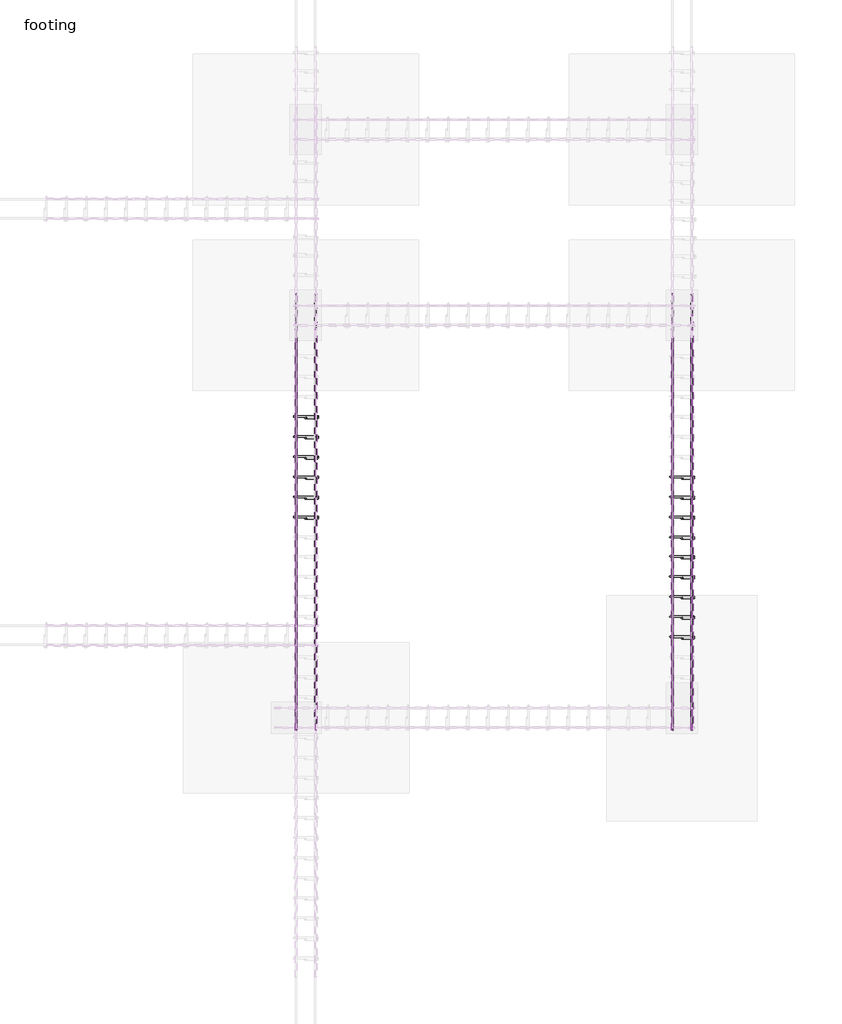
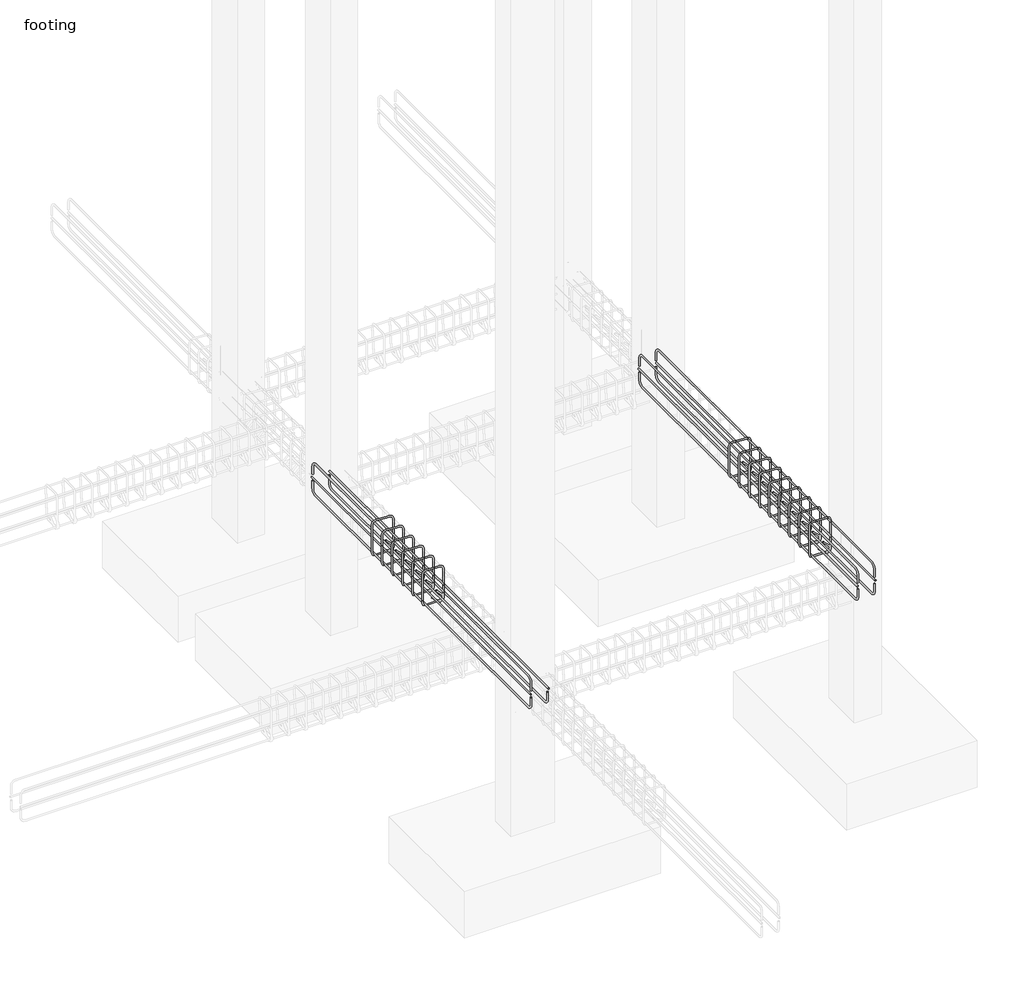
# One storey, part 12 of 21: 26 reinforcing bars.
"""IFC4 building model written with IfcOpenShell, lengths in millimetres."""

from ifc_helpers import new_model, si_unit, point, frame, origin, place, context, project, spatial, polyline, circle_curve, trimmed, segment, composite_curve, element, save
from ifc_brep_helpers import swept_disk

model = new_model("IFC4")

# Units and contexts
model_context = context("Model", 3, world=origin())
ifc_project = project(units=[si_unit("LENGTHUNIT", "METRE", prefix="MILLI")], contexts=[model_context])

# Site, building, storey
site = spatial("IfcSite", under=ifc_project)
building = spatial("IfcBuilding", under=site)
storey = spatial("IfcBuildingStorey", under=building, Name="footing", Elevation=-1524.0)

# Reinforcing bars
placement = place(None, origin())
element("IfcReinforcingBar", 1, at=placement, inside=storey, context=model_context, shape_type="SolidModel", body=[
    swept_disk(composite_curve([segment(polyline([(-7943.5663014, 3342.0730744, -170.2827408), (-7943.5663014, 3342.0730744, -94.0827408)]), True, "CONTINUOUS"), segment(trimmed(circle_curve(frame((-7943.5663014, 3386.5230744, -94.0827408), z_axis=(-1.0, 0.0, 0.0), x_axis=(0.0, -44.44999999999982, 0.0)), 44.45), [point((-7943.5663014, 3342.0730744, -94.0827408))], [point((-7943.5663014, 3386.5230744, -49.6327408))], True, "CARTESIAN"), True, "CONTINUOUS"), segment(polyline([(-7943.5663014, 3386.5230744, -49.6327408), (-7943.5663014, 6822.6668244, -49.6327408)]), True, "CONTINUOUS"), segment(trimmed(circle_curve(frame((-7943.5663014, 6822.6668244, -94.0827408), z_axis=(-1.0, 0.0, 0.0), x_axis=(0.0, 0.0, 44.449999999999996)), 44.45), [point((-7943.5663014, 6822.6668244, -49.6327408))], [point((-7943.5663014, 6867.1168244, -94.0827408))], True, "CARTESIAN"), True, "CONTINUOUS"), segment(polyline([(-7943.5663014, 6867.1168244, -94.0827408), (-7943.5663014, 6867.1168244, -170.2827408)]), True, "CONTINUOUS")], self_intersect=False), 6.35),
])
element("IfcReinforcingBar", 2, at=placement, inside=storey, context=model_context, shape_type="SolidModel", body=[
    swept_disk(composite_curve([segment(polyline([(-7788.8317831, 3342.0730744, -236.1172592), (-7788.8317831, 3342.0730744, -312.3172592)]), True, "CONTINUOUS"), segment(trimmed(circle_curve(frame((-7788.8317831, 3386.5230744, -312.3172592), z_axis=(1.0, 0.0, 0.0), x_axis=(0.0, -44.44999999999982, 0.0)), 44.45), [point((-7788.8317831, 3342.0730744, -312.3172592))], [point((-7788.8317831, 3386.5230744, -356.7672592))], True, "CARTESIAN"), True, "CONTINUOUS"), segment(polyline([(-7788.8317831, 3386.5230744, -356.7672592), (-7788.8317831, 6822.6668244, -356.7672592)]), True, "CONTINUOUS"), segment(trimmed(circle_curve(frame((-7788.8317831, 6822.6668244, -312.3172592), z_axis=(1.0, 0.0, 0.0), x_axis=(0.0, 0.0, -44.44999999999999)), 44.45), [point((-7788.8317831, 6822.6668244, -356.7672592))], [point((-7788.8317831, 6867.1168244, -312.3172592))], True, "CARTESIAN"), True, "CONTINUOUS"), segment(polyline([(-7788.8317831, 6867.1168244, -312.3172592), (-7788.8317831, 6867.1168244, -236.1172592)]), True, "CONTINUOUS")], self_intersect=False), 6.35),
])
element("IfcReinforcingBar", 3, at=placement, inside=storey, context=model_context, shape_type="SolidModel", body=[
    swept_disk(composite_curve([segment(polyline([(-7943.5663014, 3342.0730744, -236.1172592), (-7943.5663014, 3342.0730744, -312.3172592)]), True, "CONTINUOUS"), segment(trimmed(circle_curve(frame((-7943.5663014, 3386.5230744, -312.3172592), z_axis=(1.0, 0.0, 0.0), x_axis=(0.0, -44.44999999999982, 0.0)), 44.45), [point((-7943.5663014, 3342.0730744, -312.3172592))], [point((-7943.5663014, 3386.5230744, -356.7672592))], True, "CARTESIAN"), True, "CONTINUOUS"), segment(polyline([(-7943.5663014, 3386.5230744, -356.7672592), (-7943.5663014, 6822.6668244, -356.7672592)]), True, "CONTINUOUS"), segment(trimmed(circle_curve(frame((-7943.5663014, 6822.6668244, -312.3172592), z_axis=(1.0, 0.0, 0.0), x_axis=(0.0, 0.0, -44.44999999999999)), 44.45), [point((-7943.5663014, 6822.6668244, -356.7672592))], [point((-7943.5663014, 6867.1168244, -312.3172592))], True, "CARTESIAN"), True, "CONTINUOUS"), segment(polyline([(-7943.5663014, 6867.1168244, -312.3172592), (-7943.5663014, 6867.1168244, -236.1172592)]), True, "CONTINUOUS")], self_intersect=False), 6.35),
])
element("IfcReinforcingBar", 4, at=placement, inside=storey, context=model_context, shape_type="SolidModel", body=[
    swept_disk(composite_curve([segment(polyline([(-7783.2521673, 3335.7230744, -203.2), (-7783.2521673, 6873.4668244, -203.2)]), True, "CONTINUOUS")], self_intersect=False), 6.35),
])
element("IfcReinforcingBar", 5, at=placement, inside=storey, context=model_context, shape_type="SolidModel", body=[
    swept_disk(composite_curve([segment(polyline([(-7949.1459173, 3335.7230744, -203.2), (-7949.1459173, 6873.4668244, -203.2)]), True, "CONTINUOUS")], self_intersect=False), 6.35),
])
element("IfcReinforcingBar", 6, at=placement, inside=storey, context=model_context, shape_type="SolidModel", body=[
    swept_disk(composite_curve([segment(polyline([(-7834.7165254, 5064.2456073, -265.9812362), (-7779.851527, 5064.2456073, -320.8462347)]), True, "CONTINUOUS"), segment(trimmed(circle_curve(frame((-7802.3021673, 5064.2456073, -343.296875), z_axis=(0.0, 1.0, 0.0), x_axis=(22.450640300000487, 0.0, 22.450640299999975)), 31.75), [point((-7779.851527, 5064.2456073, -320.8462347))], [point((-7802.3021673, 5064.2456073, -375.046875))], True, "CARTESIAN"), True, "CONTINUOUS"), segment(polyline([(-7802.3021673, 5064.2456073, -375.046875), (-7930.0959173, 5064.2456073, -375.046875)]), True, "CONTINUOUS"), segment(trimmed(circle_curve(frame((-7930.0959173, 5064.2456073, -343.296875), z_axis=(0.0, 1.0, 0.0), x_axis=(0.0, 0.0, -31.75)), 31.75), [point((-7930.0959173, 5064.2456073, -375.046875))], [point((-7961.8459173, 5064.2456073, -343.296875))], True, "CARTESIAN"), True, "CONTINUOUS"), segment(polyline([(-7961.8459173, 5064.2456073, -343.296875), (-7961.8459173, 5064.2456073, -63.103125)]), True, "CONTINUOUS"), segment(trimmed(circle_curve(frame((-7930.165658, 5062.1423536, -63.103125), z_axis=(0.0662442117686417, 0.9978034397651431, 0.0), x_axis=(-31.680259300000216, 2.1032537000000957, 0.0)), 31.75), [point((-7961.8459173, 5064.2456073, -63.103125))], [point((-7930.165658, 5062.1423536, -31.353125))], True, "CARTESIAN"), True, "CONTINUOUS"), segment(polyline([(-7930.165658, 5062.1423536, -31.353125), (-7802.2324265, 5053.648861, -31.353125)]), True, "CONTINUOUS"), segment(trimmed(circle_curve(frame((-7802.2324265, 5053.648861, -63.103125), z_axis=(0.06624421176864169, 0.997803439765143, 0.0), x_axis=(0.0, 0.0, 31.75)), 31.75), [point((-7802.2324265, 5053.648861, -31.353125))], [point((-7770.5521673, 5051.5456073, -63.103125))], True, "CARTESIAN"), True, "CONTINUOUS"), segment(polyline([(-7770.5521673, 5051.5456073, -63.103125), (-7770.5521673, 5051.5456073, -343.296875)]), True, "CONTINUOUS"), segment(trimmed(circle_curve(frame((-7802.3021673, 5051.5456073, -343.296875), z_axis=(0.0, 1.0, 0.0), x_axis=(31.75, 0.0, 0.0)), 31.75), [point((-7770.5521673, 5051.5456073, -343.296875))], [point((-7824.7528076, 5051.5456073, -365.7475153))], True, "CARTESIAN"), True, "CONTINUOUS"), segment(polyline([(-7824.7528076, 5051.5456073, -365.7475153), (-7879.617806, 5051.5456073, -310.8825168)]), True, "CONTINUOUS")], self_intersect=False), 6.35),
])
element("IfcReinforcingBar", 7, at=placement, inside=storey, context=model_context, shape_type="SolidModel", body=[
    swept_disk(composite_curve([segment(polyline([(-7834.7165254, 5226.9456073, -265.9812362), (-7779.851527, 5226.9456073, -320.8462347)]), True, "CONTINUOUS"), segment(trimmed(circle_curve(frame((-7802.3021673, 5226.9456073, -343.296875), z_axis=(0.0, 1.0, 0.0), x_axis=(22.450640300000487, 0.0, 22.450640299999975)), 31.75), [point((-7779.851527, 5226.9456073, -320.8462347))], [point((-7802.3021673, 5226.9456073, -375.046875))], True, "CARTESIAN"), True, "CONTINUOUS"), segment(polyline([(-7802.3021673, 5226.9456073, -375.046875), (-7930.0959173, 5226.9456073, -375.046875)]), True, "CONTINUOUS"), segment(trimmed(circle_curve(frame((-7930.0959173, 5226.9456073, -343.296875), z_axis=(0.0, 1.0, 0.0), x_axis=(0.0, 0.0, -31.75)), 31.75), [point((-7930.0959173, 5226.9456073, -375.046875))], [point((-7961.8459173, 5226.9456073, -343.296875))], True, "CARTESIAN"), True, "CONTINUOUS"), segment(polyline([(-7961.8459173, 5226.9456073, -343.296875), (-7961.8459173, 5226.9456073, -63.103125)]), True, "CONTINUOUS"), segment(trimmed(circle_curve(frame((-7930.165658, 5224.8423536, -63.103125), z_axis=(0.0662442117686417, 0.9978034397651431, 0.0), x_axis=(-31.680259300000216, 2.1032537000000957, 0.0)), 31.75), [point((-7961.8459173, 5226.9456073, -63.103125))], [point((-7930.165658, 5224.8423536, -31.353125))], True, "CARTESIAN"), True, "CONTINUOUS"), segment(polyline([(-7930.165658, 5224.8423536, -31.353125), (-7802.2324265, 5216.348861, -31.353125)]), True, "CONTINUOUS"), segment(trimmed(circle_curve(frame((-7802.2324265, 5216.348861, -63.103125), z_axis=(0.06624421176864169, 0.997803439765143, 0.0), x_axis=(0.0, 0.0, 31.75)), 31.75), [point((-7802.2324265, 5216.348861, -31.353125))], [point((-7770.5521673, 5214.2456073, -63.103125))], True, "CARTESIAN"), True, "CONTINUOUS"), segment(polyline([(-7770.5521673, 5214.2456073, -63.103125), (-7770.5521673, 5214.2456073, -343.296875)]), True, "CONTINUOUS"), segment(trimmed(circle_curve(frame((-7802.3021673, 5214.2456073, -343.296875), z_axis=(0.0, 1.0, 0.0), x_axis=(31.75, 0.0, 0.0)), 31.75), [point((-7770.5521673, 5214.2456073, -343.296875))], [point((-7824.7528076, 5214.2456073, -365.7475153))], True, "CARTESIAN"), True, "CONTINUOUS"), segment(polyline([(-7824.7528076, 5214.2456073, -365.7475153), (-7879.617806, 5214.2456073, -310.8825168)]), True, "CONTINUOUS")], self_intersect=False), 6.35),
])
element("IfcReinforcingBar", 8, at=placement, inside=storey, context=model_context, shape_type="SolidModel", body=[
    swept_disk(composite_curve([segment(polyline([(-7834.7165254, 5389.6456073, -265.9812362), (-7779.851527, 5389.6456073, -320.8462347)]), True, "CONTINUOUS"), segment(trimmed(circle_curve(frame((-7802.3021673, 5389.6456073, -343.296875), z_axis=(0.0, 1.0, 0.0), x_axis=(22.450640300000487, 0.0, 22.450640299999975)), 31.75), [point((-7779.851527, 5389.6456073, -320.8462347))], [point((-7802.3021673, 5389.6456073, -375.046875))], True, "CARTESIAN"), True, "CONTINUOUS"), segment(polyline([(-7802.3021673, 5389.6456073, -375.046875), (-7930.0959173, 5389.6456073, -375.046875)]), True, "CONTINUOUS"), segment(trimmed(circle_curve(frame((-7930.0959173, 5389.6456073, -343.296875), z_axis=(0.0, 1.0, 0.0), x_axis=(0.0, 0.0, -31.75)), 31.75), [point((-7930.0959173, 5389.6456073, -375.046875))], [point((-7961.8459173, 5389.6456073, -343.296875))], True, "CARTESIAN"), True, "CONTINUOUS"), segment(polyline([(-7961.8459173, 5389.6456073, -343.296875), (-7961.8459173, 5389.6456073, -63.103125)]), True, "CONTINUOUS"), segment(trimmed(circle_curve(frame((-7930.165658, 5387.5423536, -63.103125), z_axis=(0.0662442117686417, 0.9978034397651431, 0.0), x_axis=(-31.680259300000216, 2.1032537000000957, 0.0)), 31.75), [point((-7961.8459173, 5389.6456073, -63.103125))], [point((-7930.165658, 5387.5423536, -31.353125))], True, "CARTESIAN"), True, "CONTINUOUS"), segment(polyline([(-7930.165658, 5387.5423536, -31.353125), (-7802.2324265, 5379.048861, -31.353125)]), True, "CONTINUOUS"), segment(trimmed(circle_curve(frame((-7802.2324265, 5379.048861, -63.103125), z_axis=(0.06624421176864169, 0.997803439765143, 0.0), x_axis=(0.0, 0.0, 31.75)), 31.75), [point((-7802.2324265, 5379.048861, -31.353125))], [point((-7770.5521673, 5376.9456073, -63.103125))], True, "CARTESIAN"), True, "CONTINUOUS"), segment(polyline([(-7770.5521673, 5376.9456073, -63.103125), (-7770.5521673, 5376.9456073, -343.296875)]), True, "CONTINUOUS"), segment(trimmed(circle_curve(frame((-7802.3021673, 5376.9456073, -343.296875), z_axis=(0.0, 1.0, 0.0), x_axis=(31.75, 0.0, 0.0)), 31.75), [point((-7770.5521673, 5376.9456073, -343.296875))], [point((-7824.7528076, 5376.9456073, -365.7475153))], True, "CARTESIAN"), True, "CONTINUOUS"), segment(polyline([(-7824.7528076, 5376.9456073, -365.7475153), (-7879.617806, 5376.9456073, -310.8825168)]), True, "CONTINUOUS")], self_intersect=False), 6.35),
])
element("IfcReinforcingBar", 9, at=placement, inside=storey, context=model_context, shape_type="SolidModel", body=[
    swept_disk(composite_curve([segment(polyline([(-7834.7165254, 5552.3456073, -265.9812362), (-7779.851527, 5552.3456073, -320.8462347)]), True, "CONTINUOUS"), segment(trimmed(circle_curve(frame((-7802.3021673, 5552.3456073, -343.296875), z_axis=(0.0, 1.0, 0.0), x_axis=(22.450640300000487, 0.0, 22.450640299999975)), 31.75), [point((-7779.851527, 5552.3456073, -320.8462347))], [point((-7802.3021673, 5552.3456073, -375.046875))], True, "CARTESIAN"), True, "CONTINUOUS"), segment(polyline([(-7802.3021673, 5552.3456073, -375.046875), (-7930.0959173, 5552.3456073, -375.046875)]), True, "CONTINUOUS"), segment(trimmed(circle_curve(frame((-7930.0959173, 5552.3456073, -343.296875), z_axis=(0.0, 1.0, 0.0), x_axis=(0.0, 0.0, -31.75)), 31.75), [point((-7930.0959173, 5552.3456073, -375.046875))], [point((-7961.8459173, 5552.3456073, -343.296875))], True, "CARTESIAN"), True, "CONTINUOUS"), segment(polyline([(-7961.8459173, 5552.3456073, -343.296875), (-7961.8459173, 5552.3456073, -63.103125)]), True, "CONTINUOUS"), segment(trimmed(circle_curve(frame((-7930.165658, 5550.2423536, -63.103125), z_axis=(0.0662442117686417, 0.9978034397651431, 0.0), x_axis=(-31.680259300000216, 2.1032537000000957, 0.0)), 31.75), [point((-7961.8459173, 5552.3456073, -63.103125))], [point((-7930.165658, 5550.2423536, -31.353125))], True, "CARTESIAN"), True, "CONTINUOUS"), segment(polyline([(-7930.165658, 5550.2423536, -31.353125), (-7802.2324265, 5541.748861, -31.353125)]), True, "CONTINUOUS"), segment(trimmed(circle_curve(frame((-7802.2324265, 5541.748861, -63.103125), z_axis=(0.06624421176864169, 0.997803439765143, 0.0), x_axis=(0.0, 0.0, 31.75)), 31.75), [point((-7802.2324265, 5541.748861, -31.353125))], [point((-7770.5521673, 5539.6456073, -63.103125))], True, "CARTESIAN"), True, "CONTINUOUS"), segment(polyline([(-7770.5521673, 5539.6456073, -63.103125), (-7770.5521673, 5539.6456073, -343.296875)]), True, "CONTINUOUS"), segment(trimmed(circle_curve(frame((-7802.3021673, 5539.6456073, -343.296875), z_axis=(0.0, 1.0, 0.0), x_axis=(31.75, 0.0, 0.0)), 31.75), [point((-7770.5521673, 5539.6456073, -343.296875))], [point((-7824.7528076, 5539.6456073, -365.7475153))], True, "CARTESIAN"), True, "CONTINUOUS"), segment(polyline([(-7824.7528076, 5539.6456073, -365.7475153), (-7879.617806, 5539.6456073, -310.8825168)]), True, "CONTINUOUS")], self_intersect=False), 6.35),
])
element("IfcReinforcingBar", 10, at=placement, inside=storey, context=model_context, shape_type="SolidModel", body=[
    swept_disk(composite_curve([segment(polyline([(-7834.7165254, 5715.0456073, -265.9812362), (-7779.851527, 5715.0456073, -320.8462347)]), True, "CONTINUOUS"), segment(trimmed(circle_curve(frame((-7802.3021673, 5715.0456073, -343.296875), z_axis=(0.0, 1.0, 0.0), x_axis=(22.450640300000487, 0.0, 22.450640299999975)), 31.75), [point((-7779.851527, 5715.0456073, -320.8462347))], [point((-7802.3021673, 5715.0456073, -375.046875))], True, "CARTESIAN"), True, "CONTINUOUS"), segment(polyline([(-7802.3021673, 5715.0456073, -375.046875), (-7930.0959173, 5715.0456073, -375.046875)]), True, "CONTINUOUS"), segment(trimmed(circle_curve(frame((-7930.0959173, 5715.0456073, -343.296875), z_axis=(0.0, 1.0, 0.0), x_axis=(0.0, 0.0, -31.75)), 31.75), [point((-7930.0959173, 5715.0456073, -375.046875))], [point((-7961.8459173, 5715.0456073, -343.296875))], True, "CARTESIAN"), True, "CONTINUOUS"), segment(polyline([(-7961.8459173, 5715.0456073, -343.296875), (-7961.8459173, 5715.0456073, -63.103125)]), True, "CONTINUOUS"), segment(trimmed(circle_curve(frame((-7930.165658, 5712.9423536, -63.103125), z_axis=(0.0662442117686417, 0.9978034397651431, 0.0), x_axis=(-31.680259300000216, 2.103253699999186, 0.0)), 31.75), [point((-7961.8459173, 5715.0456073, -63.103125))], [point((-7930.165658, 5712.9423536, -31.353125))], True, "CARTESIAN"), True, "CONTINUOUS"), segment(polyline([(-7930.165658, 5712.9423536, -31.353125), (-7802.2324265, 5704.448861, -31.353125)]), True, "CONTINUOUS"), segment(trimmed(circle_curve(frame((-7802.2324265, 5704.448861, -63.103125), z_axis=(0.06624421176864169, 0.997803439765143, 0.0), x_axis=(0.0, 0.0, 31.75)), 31.75), [point((-7802.2324265, 5704.448861, -31.353125))], [point((-7770.5521673, 5702.3456073, -63.103125))], True, "CARTESIAN"), True, "CONTINUOUS"), segment(polyline([(-7770.5521673, 5702.3456073, -63.103125), (-7770.5521673, 5702.3456073, -343.296875)]), True, "CONTINUOUS"), segment(trimmed(circle_curve(frame((-7802.3021673, 5702.3456073, -343.296875), z_axis=(0.0, 1.0, 0.0), x_axis=(31.75, 0.0, 0.0)), 31.75), [point((-7770.5521673, 5702.3456073, -343.296875))], [point((-7824.7528076, 5702.3456073, -365.7475153))], True, "CARTESIAN"), True, "CONTINUOUS"), segment(polyline([(-7824.7528076, 5702.3456073, -365.7475153), (-7879.617806, 5702.3456073, -310.8825168)]), True, "CONTINUOUS")], self_intersect=False), 6.35),
])
element("IfcReinforcingBar", 11, at=placement, inside=storey, context=model_context, shape_type="SolidModel", body=[
    swept_disk(composite_curve([segment(polyline([(-7834.7165254, 5877.7456073, -265.9812362), (-7779.851527, 5877.7456073, -320.8462347)]), True, "CONTINUOUS"), segment(trimmed(circle_curve(frame((-7802.3021673, 5877.7456073, -343.296875), z_axis=(0.0, 1.0, 0.0), x_axis=(22.450640300000487, 0.0, 22.450640299999975)), 31.75), [point((-7779.851527, 5877.7456073, -320.8462347))], [point((-7802.3021673, 5877.7456073, -375.046875))], True, "CARTESIAN"), True, "CONTINUOUS"), segment(polyline([(-7802.3021673, 5877.7456073, -375.046875), (-7930.0959173, 5877.7456073, -375.046875)]), True, "CONTINUOUS"), segment(trimmed(circle_curve(frame((-7930.0959173, 5877.7456073, -343.296875), z_axis=(0.0, 1.0, 0.0), x_axis=(0.0, 0.0, -31.75)), 31.75), [point((-7930.0959173, 5877.7456073, -375.046875))], [point((-7961.8459173, 5877.7456073, -343.296875))], True, "CARTESIAN"), True, "CONTINUOUS"), segment(polyline([(-7961.8459173, 5877.7456073, -343.296875), (-7961.8459173, 5877.7456073, -63.103125)]), True, "CONTINUOUS"), segment(trimmed(circle_curve(frame((-7930.165658, 5875.6423536, -63.103125), z_axis=(0.0662442117686417, 0.9978034397651431, 0.0), x_axis=(-31.680259300000216, 2.1032537000000957, 0.0)), 31.75), [point((-7961.8459173, 5877.7456073, -63.103125))], [point((-7930.165658, 5875.6423536, -31.353125))], True, "CARTESIAN"), True, "CONTINUOUS"), segment(polyline([(-7930.165658, 5875.6423536, -31.353125), (-7802.2324265, 5867.148861, -31.353125)]), True, "CONTINUOUS"), segment(trimmed(circle_curve(frame((-7802.2324265, 5867.148861, -63.103125), z_axis=(0.06624421176864169, 0.997803439765143, 0.0), x_axis=(0.0, 0.0, 31.75)), 31.75), [point((-7802.2324265, 5867.148861, -31.353125))], [point((-7770.5521673, 5865.0456073, -63.103125))], True, "CARTESIAN"), True, "CONTINUOUS"), segment(polyline([(-7770.5521673, 5865.0456073, -63.103125), (-7770.5521673, 5865.0456073, -343.296875)]), True, "CONTINUOUS"), segment(trimmed(circle_curve(frame((-7802.3021673, 5865.0456073, -343.296875), z_axis=(0.0, 1.0, 0.0), x_axis=(31.75, 0.0, 0.0)), 31.75), [point((-7770.5521673, 5865.0456073, -343.296875))], [point((-7824.7528076, 5865.0456073, -365.7475153))], True, "CARTESIAN"), True, "CONTINUOUS"), segment(polyline([(-7824.7528076, 5865.0456073, -365.7475153), (-7879.617806, 5865.0456073, -310.8825168)]), True, "CONTINUOUS")], self_intersect=False), 6.35),
])
element("IfcReinforcingBar", 12, at=placement, inside=storey, context=model_context, shape_type="SolidModel", body=[
    swept_disk(composite_curve([segment(polyline([(-4740.8317831, 3342.0730744, -170.2827408), (-4740.8317831, 3342.0730744, -94.0827408)]), True, "CONTINUOUS"), segment(trimmed(circle_curve(frame((-4740.8317831, 3386.5230744, -94.0827408), z_axis=(-1.0, 0.0, 0.0), x_axis=(0.0, -44.44999999999982, 0.0)), 44.45), [point((-4740.8317831, 3342.0730744, -94.0827408))], [point((-4740.8317831, 3386.5230744, -49.6327408))], True, "CARTESIAN"), True, "CONTINUOUS"), segment(polyline([(-4740.8317831, 3386.5230744, -49.6327408), (-4740.8317831, 6822.6668244, -49.6327408)]), True, "CONTINUOUS"), segment(trimmed(circle_curve(frame((-4740.8317831, 6822.6668244, -94.0827408), z_axis=(-1.0, 0.0, 0.0), x_axis=(0.0, 0.0, 44.449999999999996)), 44.45), [point((-4740.8317831, 6822.6668244, -49.6327408))], [point((-4740.8317831, 6867.1168244, -94.0827408))], True, "CARTESIAN"), True, "CONTINUOUS"), segment(polyline([(-4740.8317831, 6867.1168244, -94.0827408), (-4740.8317831, 6867.1168244, -170.2827408)]), True, "CONTINUOUS")], self_intersect=False), 6.35),
])
element("IfcReinforcingBar", 13, at=placement, inside=storey, context=model_context, shape_type="SolidModel", body=[
    swept_disk(composite_curve([segment(polyline([(-4895.5663014, 3342.0730744, -170.2827408), (-4895.5663014, 3342.0730744, -94.0827408)]), True, "CONTINUOUS"), segment(trimmed(circle_curve(frame((-4895.5663014, 3386.5230744, -94.0827408), z_axis=(-1.0, 0.0, 0.0), x_axis=(0.0, -44.44999999999982, 0.0)), 44.45), [point((-4895.5663014, 3342.0730744, -94.0827408))], [point((-4895.5663014, 3386.5230744, -49.6327408))], True, "CARTESIAN"), True, "CONTINUOUS"), segment(polyline([(-4895.5663014, 3386.5230744, -49.6327408), (-4895.5663014, 6822.6668244, -49.6327408)]), True, "CONTINUOUS"), segment(trimmed(circle_curve(frame((-4895.5663014, 6822.6668244, -94.0827408), z_axis=(-1.0, 0.0, 0.0), x_axis=(0.0, 0.0, 44.449999999999996)), 44.45), [point((-4895.5663014, 6822.6668244, -49.6327408))], [point((-4895.5663014, 6867.1168244, -94.0827408))], True, "CARTESIAN"), True, "CONTINUOUS"), segment(polyline([(-4895.5663014, 6867.1168244, -94.0827408), (-4895.5663014, 6867.1168244, -170.2827408)]), True, "CONTINUOUS")], self_intersect=False), 6.35),
])
element("IfcReinforcingBar", 14, at=placement, inside=storey, context=model_context, shape_type="SolidModel", body=[
    swept_disk(composite_curve([segment(polyline([(-4740.8317831, 3342.0730744, -236.1172592), (-4740.8317831, 3342.0730744, -312.3172592)]), True, "CONTINUOUS"), segment(trimmed(circle_curve(frame((-4740.8317831, 3386.5230744, -312.3172592), z_axis=(1.0, 0.0, 0.0), x_axis=(0.0, -44.44999999999982, 0.0)), 44.45), [point((-4740.8317831, 3342.0730744, -312.3172592))], [point((-4740.8317831, 3386.5230744, -356.7672592))], True, "CARTESIAN"), True, "CONTINUOUS"), segment(polyline([(-4740.8317831, 3386.5230744, -356.7672592), (-4740.8317831, 6822.6668244, -356.7672592)]), True, "CONTINUOUS"), segment(trimmed(circle_curve(frame((-4740.8317831, 6822.6668244, -312.3172592), z_axis=(1.0, 0.0, 0.0), x_axis=(0.0, 0.0, -44.44999999999999)), 44.45), [point((-4740.8317831, 6822.6668244, -356.7672592))], [point((-4740.8317831, 6867.1168244, -312.3172592))], True, "CARTESIAN"), True, "CONTINUOUS"), segment(polyline([(-4740.8317831, 6867.1168244, -312.3172592), (-4740.8317831, 6867.1168244, -236.1172592)]), True, "CONTINUOUS")], self_intersect=False), 6.35),
])
element("IfcReinforcingBar", 15, at=placement, inside=storey, context=model_context, shape_type="SolidModel", body=[
    swept_disk(composite_curve([segment(polyline([(-4895.5663014, 3342.0730744, -236.1172592), (-4895.5663014, 3342.0730744, -312.3172592)]), True, "CONTINUOUS"), segment(trimmed(circle_curve(frame((-4895.5663014, 3386.5230744, -312.3172592), z_axis=(1.0, 0.0, 0.0), x_axis=(0.0, -44.44999999999982, 0.0)), 44.45), [point((-4895.5663014, 3342.0730744, -312.3172592))], [point((-4895.5663014, 3386.5230744, -356.7672592))], True, "CARTESIAN"), True, "CONTINUOUS"), segment(polyline([(-4895.5663014, 3386.5230744, -356.7672592), (-4895.5663014, 6822.6668244, -356.7672592)]), True, "CONTINUOUS"), segment(trimmed(circle_curve(frame((-4895.5663014, 6822.6668244, -312.3172592), z_axis=(1.0, 0.0, 0.0), x_axis=(0.0, 0.0, -44.44999999999999)), 44.45), [point((-4895.5663014, 6822.6668244, -356.7672592))], [point((-4895.5663014, 6867.1168244, -312.3172592))], True, "CARTESIAN"), True, "CONTINUOUS"), segment(polyline([(-4895.5663014, 6867.1168244, -312.3172592), (-4895.5663014, 6867.1168244, -236.1172592)]), True, "CONTINUOUS")], self_intersect=False), 6.35),
])
element("IfcReinforcingBar", 16, at=placement, inside=storey, context=model_context, shape_type="SolidModel", body=[
    swept_disk(composite_curve([segment(polyline([(-4735.2521673, 3335.7230744, -203.2), (-4735.2521673, 6873.4668244, -203.2)]), True, "CONTINUOUS")], self_intersect=False), 6.35),
])
element("IfcReinforcingBar", 17, at=placement, inside=storey, context=model_context, shape_type="SolidModel", body=[
    swept_disk(composite_curve([segment(polyline([(-4901.1459173, 3335.7230744, -203.2), (-4901.1459173, 6873.4668244, -203.2)]), True, "CONTINUOUS")], self_intersect=False), 6.35),
])
element("IfcReinforcingBar", 18, at=placement, inside=storey, context=model_context, shape_type="SolidModel", body=[
    swept_disk(composite_curve([segment(polyline([(-4786.7165254, 4094.3956073, -265.9812362), (-4731.851527, 4094.3956073, -320.8462347)]), True, "CONTINUOUS"), segment(trimmed(circle_curve(frame((-4754.3021673, 4094.3956073, -343.296875), z_axis=(0.0, 1.0, 0.0), x_axis=(22.450640300000487, 0.0, 22.450640299999975)), 31.75), [point((-4731.851527, 4094.3956073, -320.8462347))], [point((-4754.3021673, 4094.3956073, -375.046875))], True, "CARTESIAN"), True, "CONTINUOUS"), segment(polyline([(-4754.3021673, 4094.3956073, -375.046875), (-4882.0959173, 4094.3956073, -375.046875)]), True, "CONTINUOUS"), segment(trimmed(circle_curve(frame((-4882.0959173, 4094.3956073, -343.296875), z_axis=(0.0, 1.0, 0.0), x_axis=(0.0, 0.0, -31.75)), 31.75), [point((-4882.0959173, 4094.3956073, -375.046875))], [point((-4913.8459173, 4094.3956073, -343.296875))], True, "CARTESIAN"), True, "CONTINUOUS"), segment(polyline([(-4913.8459173, 4094.3956073, -343.296875), (-4913.8459173, 4094.3956073, -63.103125)]), True, "CONTINUOUS"), segment(trimmed(circle_curve(frame((-4882.165658, 4092.2923536, -63.103125), z_axis=(0.0662442117686417, 0.9978034397651431, 0.0), x_axis=(-31.680259300000216, 2.1032537000000957, 0.0)), 31.75), [point((-4913.8459173, 4094.3956073, -63.103125))], [point((-4882.165658, 4092.2923536, -31.353125))], True, "CARTESIAN"), True, "CONTINUOUS"), segment(polyline([(-4882.165658, 4092.2923536, -31.353125), (-4754.2324265, 4083.798861, -31.353125)]), True, "CONTINUOUS"), segment(trimmed(circle_curve(frame((-4754.2324265, 4083.798861, -63.103125), z_axis=(0.06624421176864169, 0.997803439765143, 0.0), x_axis=(0.0, 0.0, 31.75)), 31.75), [point((-4754.2324265, 4083.798861, -31.353125))], [point((-4722.5521673, 4081.6956073, -63.103125))], True, "CARTESIAN"), True, "CONTINUOUS"), segment(polyline([(-4722.5521673, 4081.6956073, -63.103125), (-4722.5521673, 4081.6956073, -343.296875)]), True, "CONTINUOUS"), segment(trimmed(circle_curve(frame((-4754.3021673, 4081.6956073, -343.296875), z_axis=(0.0, 1.0, 0.0), x_axis=(31.75, 0.0, 0.0)), 31.75), [point((-4722.5521673, 4081.6956073, -343.296875))], [point((-4776.7528076, 4081.6956073, -365.7475153))], True, "CARTESIAN"), True, "CONTINUOUS"), segment(polyline([(-4776.7528076, 4081.6956073, -365.7475153), (-4831.617806, 4081.6956073, -310.8825168)]), True, "CONTINUOUS")], self_intersect=False), 6.35),
])
element("IfcReinforcingBar", 19, at=placement, inside=storey, context=model_context, shape_type="SolidModel", body=[
    swept_disk(composite_curve([segment(polyline([(-4786.7165254, 4257.0956073, -265.9812362), (-4731.851527, 4257.0956073, -320.8462347)]), True, "CONTINUOUS"), segment(trimmed(circle_curve(frame((-4754.3021673, 4257.0956073, -343.296875), z_axis=(0.0, 1.0, 0.0), x_axis=(22.450640300000487, 0.0, 22.450640299999975)), 31.75), [point((-4731.851527, 4257.0956073, -320.8462347))], [point((-4754.3021673, 4257.0956073, -375.046875))], True, "CARTESIAN"), True, "CONTINUOUS"), segment(polyline([(-4754.3021673, 4257.0956073, -375.046875), (-4882.0959173, 4257.0956073, -375.046875)]), True, "CONTINUOUS"), segment(trimmed(circle_curve(frame((-4882.0959173, 4257.0956073, -343.296875), z_axis=(0.0, 1.0, 0.0), x_axis=(0.0, 0.0, -31.75)), 31.75), [point((-4882.0959173, 4257.0956073, -375.046875))], [point((-4913.8459173, 4257.0956073, -343.296875))], True, "CARTESIAN"), True, "CONTINUOUS"), segment(polyline([(-4913.8459173, 4257.0956073, -343.296875), (-4913.8459173, 4257.0956073, -63.103125)]), True, "CONTINUOUS"), segment(trimmed(circle_curve(frame((-4882.165658, 4254.9923536, -63.103125), z_axis=(0.0662442117686417, 0.9978034397651431, 0.0), x_axis=(-31.680259300000216, 2.1032537000000957, 0.0)), 31.75), [point((-4913.8459173, 4257.0956073, -63.103125))], [point((-4882.165658, 4254.9923536, -31.353125))], True, "CARTESIAN"), True, "CONTINUOUS"), segment(polyline([(-4882.165658, 4254.9923536, -31.353125), (-4754.2324265, 4246.498861, -31.353125)]), True, "CONTINUOUS"), segment(trimmed(circle_curve(frame((-4754.2324265, 4246.498861, -63.103125), z_axis=(0.06624421176864169, 0.997803439765143, 0.0), x_axis=(0.0, 0.0, 31.75)), 31.75), [point((-4754.2324265, 4246.498861, -31.353125))], [point((-4722.5521673, 4244.3956073, -63.103125))], True, "CARTESIAN"), True, "CONTINUOUS"), segment(polyline([(-4722.5521673, 4244.3956073, -63.103125), (-4722.5521673, 4244.3956073, -343.296875)]), True, "CONTINUOUS"), segment(trimmed(circle_curve(frame((-4754.3021673, 4244.3956073, -343.296875), z_axis=(0.0, 1.0, 0.0), x_axis=(31.75, 0.0, 0.0)), 31.75), [point((-4722.5521673, 4244.3956073, -343.296875))], [point((-4776.7528076, 4244.3956073, -365.7475153))], True, "CARTESIAN"), True, "CONTINUOUS"), segment(polyline([(-4776.7528076, 4244.3956073, -365.7475153), (-4831.617806, 4244.3956073, -310.8825168)]), True, "CONTINUOUS")], self_intersect=False), 6.35),
])
element("IfcReinforcingBar", 20, at=placement, inside=storey, context=model_context, shape_type="SolidModel", body=[
    swept_disk(composite_curve([segment(polyline([(-4786.7165254, 4419.7956073, -265.9812362), (-4731.851527, 4419.7956073, -320.8462347)]), True, "CONTINUOUS"), segment(trimmed(circle_curve(frame((-4754.3021673, 4419.7956073, -343.296875), z_axis=(0.0, 1.0, 0.0), x_axis=(22.450640300000487, 0.0, 22.450640299999975)), 31.75), [point((-4731.851527, 4419.7956073, -320.8462347))], [point((-4754.3021673, 4419.7956073, -375.046875))], True, "CARTESIAN"), True, "CONTINUOUS"), segment(polyline([(-4754.3021673, 4419.7956073, -375.046875), (-4882.0959173, 4419.7956073, -375.046875)]), True, "CONTINUOUS"), segment(trimmed(circle_curve(frame((-4882.0959173, 4419.7956073, -343.296875), z_axis=(0.0, 1.0, 0.0), x_axis=(0.0, 0.0, -31.75)), 31.75), [point((-4882.0959173, 4419.7956073, -375.046875))], [point((-4913.8459173, 4419.7956073, -343.296875))], True, "CARTESIAN"), True, "CONTINUOUS"), segment(polyline([(-4913.8459173, 4419.7956073, -343.296875), (-4913.8459173, 4419.7956073, -63.103125)]), True, "CONTINUOUS"), segment(trimmed(circle_curve(frame((-4882.165658, 4417.6923536, -63.103125), z_axis=(0.0662442117686417, 0.9978034397651431, 0.0), x_axis=(-31.680259300000216, 2.103253699999186, 0.0)), 31.75), [point((-4913.8459173, 4419.7956073, -63.103125))], [point((-4882.165658, 4417.6923536, -31.353125))], True, "CARTESIAN"), True, "CONTINUOUS"), segment(polyline([(-4882.165658, 4417.6923536, -31.353125), (-4754.2324265, 4409.198861, -31.353125)]), True, "CONTINUOUS"), segment(trimmed(circle_curve(frame((-4754.2324265, 4409.198861, -63.103125), z_axis=(0.06624421176864169, 0.997803439765143, 0.0), x_axis=(0.0, 0.0, 31.75)), 31.75), [point((-4754.2324265, 4409.198861, -31.353125))], [point((-4722.5521673, 4407.0956073, -63.103125))], True, "CARTESIAN"), True, "CONTINUOUS"), segment(polyline([(-4722.5521673, 4407.0956073, -63.103125), (-4722.5521673, 4407.0956073, -343.296875)]), True, "CONTINUOUS"), segment(trimmed(circle_curve(frame((-4754.3021673, 4407.0956073, -343.296875), z_axis=(0.0, 1.0, 0.0), x_axis=(31.75, 0.0, 0.0)), 31.75), [point((-4722.5521673, 4407.0956073, -343.296875))], [point((-4776.7528076, 4407.0956073, -365.7475153))], True, "CARTESIAN"), True, "CONTINUOUS"), segment(polyline([(-4776.7528076, 4407.0956073, -365.7475153), (-4831.617806, 4407.0956073, -310.8825168)]), True, "CONTINUOUS")], self_intersect=False), 6.35),
])
element("IfcReinforcingBar", 21, at=placement, inside=storey, context=model_context, shape_type="SolidModel", body=[
    swept_disk(composite_curve([segment(polyline([(-4786.7165254, 4582.4956073, -265.9812362), (-4731.851527, 4582.4956073, -320.8462347)]), True, "CONTINUOUS"), segment(trimmed(circle_curve(frame((-4754.3021673, 4582.4956073, -343.296875), z_axis=(0.0, 1.0, 0.0), x_axis=(22.450640300000487, 0.0, 22.450640299999975)), 31.75), [point((-4731.851527, 4582.4956073, -320.8462347))], [point((-4754.3021673, 4582.4956073, -375.046875))], True, "CARTESIAN"), True, "CONTINUOUS"), segment(polyline([(-4754.3021673, 4582.4956073, -375.046875), (-4882.0959173, 4582.4956073, -375.046875)]), True, "CONTINUOUS"), segment(trimmed(circle_curve(frame((-4882.0959173, 4582.4956073, -343.296875), z_axis=(0.0, 1.0, 0.0), x_axis=(0.0, 0.0, -31.75)), 31.75), [point((-4882.0959173, 4582.4956073, -375.046875))], [point((-4913.8459173, 4582.4956073, -343.296875))], True, "CARTESIAN"), True, "CONTINUOUS"), segment(polyline([(-4913.8459173, 4582.4956073, -343.296875), (-4913.8459173, 4582.4956073, -63.103125)]), True, "CONTINUOUS"), segment(trimmed(circle_curve(frame((-4882.165658, 4580.3923536, -63.103125), z_axis=(0.0662442117686417, 0.9978034397651431, 0.0), x_axis=(-31.680259300000216, 2.1032537000000957, 0.0)), 31.75), [point((-4913.8459173, 4582.4956073, -63.103125))], [point((-4882.165658, 4580.3923536, -31.353125))], True, "CARTESIAN"), True, "CONTINUOUS"), segment(polyline([(-4882.165658, 4580.3923536, -31.353125), (-4754.2324265, 4571.898861, -31.353125)]), True, "CONTINUOUS"), segment(trimmed(circle_curve(frame((-4754.2324265, 4571.898861, -63.103125), z_axis=(0.06624421176864169, 0.997803439765143, 0.0), x_axis=(0.0, 0.0, 31.75)), 31.75), [point((-4754.2324265, 4571.898861, -31.353125))], [point((-4722.5521673, 4569.7956073, -63.103125))], True, "CARTESIAN"), True, "CONTINUOUS"), segment(polyline([(-4722.5521673, 4569.7956073, -63.103125), (-4722.5521673, 4569.7956073, -343.296875)]), True, "CONTINUOUS"), segment(trimmed(circle_curve(frame((-4754.3021673, 4569.7956073, -343.296875), z_axis=(0.0, 1.0, 0.0), x_axis=(31.75, 0.0, 0.0)), 31.75), [point((-4722.5521673, 4569.7956073, -343.296875))], [point((-4776.7528076, 4569.7956073, -365.7475153))], True, "CARTESIAN"), True, "CONTINUOUS"), segment(polyline([(-4776.7528076, 4569.7956073, -365.7475153), (-4831.617806, 4569.7956073, -310.8825168)]), True, "CONTINUOUS")], self_intersect=False), 6.35),
])
element("IfcReinforcingBar", 22, at=placement, inside=storey, context=model_context, shape_type="SolidModel", body=[
    swept_disk(composite_curve([segment(polyline([(-4786.7165254, 4745.1956073, -265.9812362), (-4731.851527, 4745.1956073, -320.8462347)]), True, "CONTINUOUS"), segment(trimmed(circle_curve(frame((-4754.3021673, 4745.1956073, -343.296875), z_axis=(0.0, 1.0, 0.0), x_axis=(22.450640300000487, 0.0, 22.450640299999975)), 31.75), [point((-4731.851527, 4745.1956073, -320.8462347))], [point((-4754.3021673, 4745.1956073, -375.046875))], True, "CARTESIAN"), True, "CONTINUOUS"), segment(polyline([(-4754.3021673, 4745.1956073, -375.046875), (-4882.0959173, 4745.1956073, -375.046875)]), True, "CONTINUOUS"), segment(trimmed(circle_curve(frame((-4882.0959173, 4745.1956073, -343.296875), z_axis=(0.0, 1.0, 0.0), x_axis=(0.0, 0.0, -31.75)), 31.75), [point((-4882.0959173, 4745.1956073, -375.046875))], [point((-4913.8459173, 4745.1956073, -343.296875))], True, "CARTESIAN"), True, "CONTINUOUS"), segment(polyline([(-4913.8459173, 4745.1956073, -343.296875), (-4913.8459173, 4745.1956073, -63.103125)]), True, "CONTINUOUS"), segment(trimmed(circle_curve(frame((-4882.165658, 4743.0923536, -63.103125), z_axis=(0.0662442117686417, 0.9978034397651431, 0.0), x_axis=(-31.680259300000216, 2.1032537000000957, 0.0)), 31.75), [point((-4913.8459173, 4745.1956073, -63.103125))], [point((-4882.165658, 4743.0923536, -31.353125))], True, "CARTESIAN"), True, "CONTINUOUS"), segment(polyline([(-4882.165658, 4743.0923536, -31.353125), (-4754.2324265, 4734.598861, -31.353125)]), True, "CONTINUOUS"), segment(trimmed(circle_curve(frame((-4754.2324265, 4734.598861, -63.103125), z_axis=(0.06624421176864169, 0.997803439765143, 0.0), x_axis=(0.0, 0.0, 31.75)), 31.75), [point((-4754.2324265, 4734.598861, -31.353125))], [point((-4722.5521673, 4732.4956073, -63.103125))], True, "CARTESIAN"), True, "CONTINUOUS"), segment(polyline([(-4722.5521673, 4732.4956073, -63.103125), (-4722.5521673, 4732.4956073, -343.296875)]), True, "CONTINUOUS"), segment(trimmed(circle_curve(frame((-4754.3021673, 4732.4956073, -343.296875), z_axis=(0.0, 1.0, 0.0), x_axis=(31.75, 0.0, 0.0)), 31.75), [point((-4722.5521673, 4732.4956073, -343.296875))], [point((-4776.7528076, 4732.4956073, -365.7475153))], True, "CARTESIAN"), True, "CONTINUOUS"), segment(polyline([(-4776.7528076, 4732.4956073, -365.7475153), (-4831.617806, 4732.4956073, -310.8825168)]), True, "CONTINUOUS")], self_intersect=False), 6.35),
])
element("IfcReinforcingBar", 23, at=placement, inside=storey, context=model_context, shape_type="SolidModel", body=[
    swept_disk(composite_curve([segment(polyline([(-4786.7165254, 4901.5456073, -265.9812362), (-4731.851527, 4901.5456073, -320.8462347)]), True, "CONTINUOUS"), segment(trimmed(circle_curve(frame((-4754.3021673, 4901.5456073, -343.296875), z_axis=(0.0, 1.0, 0.0), x_axis=(22.450640300000487, 0.0, 22.450640299999975)), 31.75), [point((-4731.851527, 4901.5456073, -320.8462347))], [point((-4754.3021673, 4901.5456073, -375.046875))], True, "CARTESIAN"), True, "CONTINUOUS"), segment(polyline([(-4754.3021673, 4901.5456073, -375.046875), (-4882.0959173, 4901.5456073, -375.046875)]), True, "CONTINUOUS"), segment(trimmed(circle_curve(frame((-4882.0959173, 4901.5456073, -343.296875), z_axis=(0.0, 1.0, 0.0), x_axis=(0.0, 0.0, -31.75)), 31.75), [point((-4882.0959173, 4901.5456073, -375.046875))], [point((-4913.8459173, 4901.5456073, -343.296875))], True, "CARTESIAN"), True, "CONTINUOUS"), segment(polyline([(-4913.8459173, 4901.5456073, -343.296875), (-4913.8459173, 4901.5456073, -63.103125)]), True, "CONTINUOUS"), segment(trimmed(circle_curve(frame((-4882.165658, 4899.4423536, -63.103125), z_axis=(0.0662442117686417, 0.9978034397651431, 0.0), x_axis=(-31.680259300000216, 2.103253699999186, 0.0)), 31.75), [point((-4913.8459173, 4901.5456073, -63.103125))], [point((-4882.165658, 4899.4423536, -31.353125))], True, "CARTESIAN"), True, "CONTINUOUS"), segment(polyline([(-4882.165658, 4899.4423536, -31.353125), (-4754.2324265, 4890.948861, -31.353125)]), True, "CONTINUOUS"), segment(trimmed(circle_curve(frame((-4754.2324265, 4890.948861, -63.103125), z_axis=(0.06624421176864169, 0.997803439765143, 0.0), x_axis=(0.0, 0.0, 31.75)), 31.75), [point((-4754.2324265, 4890.948861, -31.353125))], [point((-4722.5521673, 4888.8456073, -63.103125))], True, "CARTESIAN"), True, "CONTINUOUS"), segment(polyline([(-4722.5521673, 4888.8456073, -63.103125), (-4722.5521673, 4888.8456073, -343.296875)]), True, "CONTINUOUS"), segment(trimmed(circle_curve(frame((-4754.3021673, 4888.8456073, -343.296875), z_axis=(0.0, 1.0, 0.0), x_axis=(31.75, 0.0, 0.0)), 31.75), [point((-4722.5521673, 4888.8456073, -343.296875))], [point((-4776.7528076, 4888.8456073, -365.7475153))], True, "CARTESIAN"), True, "CONTINUOUS"), segment(polyline([(-4776.7528076, 4888.8456073, -365.7475153), (-4831.617806, 4888.8456073, -310.8825168)]), True, "CONTINUOUS")], self_intersect=False), 6.35),
])
element("IfcReinforcingBar", 24, at=placement, inside=storey, context=model_context, shape_type="SolidModel", body=[
    swept_disk(composite_curve([segment(polyline([(-4786.7165254, 5064.2456073, -265.9812362), (-4731.851527, 5064.2456073, -320.8462347)]), True, "CONTINUOUS"), segment(trimmed(circle_curve(frame((-4754.3021673, 5064.2456073, -343.296875), z_axis=(0.0, 1.0, 0.0), x_axis=(22.450640300000487, 0.0, 22.450640299999975)), 31.75), [point((-4731.851527, 5064.2456073, -320.8462347))], [point((-4754.3021673, 5064.2456073, -375.046875))], True, "CARTESIAN"), True, "CONTINUOUS"), segment(polyline([(-4754.3021673, 5064.2456073, -375.046875), (-4882.0959173, 5064.2456073, -375.046875)]), True, "CONTINUOUS"), segment(trimmed(circle_curve(frame((-4882.0959173, 5064.2456073, -343.296875), z_axis=(0.0, 1.0, 0.0), x_axis=(0.0, 0.0, -31.75)), 31.75), [point((-4882.0959173, 5064.2456073, -375.046875))], [point((-4913.8459173, 5064.2456073, -343.296875))], True, "CARTESIAN"), True, "CONTINUOUS"), segment(polyline([(-4913.8459173, 5064.2456073, -343.296875), (-4913.8459173, 5064.2456073, -63.103125)]), True, "CONTINUOUS"), segment(trimmed(circle_curve(frame((-4882.165658, 5062.1423536, -63.103125), z_axis=(0.0662442117686417, 0.9978034397651431, 0.0), x_axis=(-31.680259300000216, 2.1032537000000957, 0.0)), 31.75), [point((-4913.8459173, 5064.2456073, -63.103125))], [point((-4882.165658, 5062.1423536, -31.353125))], True, "CARTESIAN"), True, "CONTINUOUS"), segment(polyline([(-4882.165658, 5062.1423536, -31.353125), (-4754.2324265, 5053.648861, -31.353125)]), True, "CONTINUOUS"), segment(trimmed(circle_curve(frame((-4754.2324265, 5053.648861, -63.103125), z_axis=(0.06624421176864169, 0.997803439765143, 0.0), x_axis=(0.0, 0.0, 31.75)), 31.75), [point((-4754.2324265, 5053.648861, -31.353125))], [point((-4722.5521673, 5051.5456073, -63.103125))], True, "CARTESIAN"), True, "CONTINUOUS"), segment(polyline([(-4722.5521673, 5051.5456073, -63.103125), (-4722.5521673, 5051.5456073, -343.296875)]), True, "CONTINUOUS"), segment(trimmed(circle_curve(frame((-4754.3021673, 5051.5456073, -343.296875), z_axis=(0.0, 1.0, 0.0), x_axis=(31.75, 0.0, 0.0)), 31.75), [point((-4722.5521673, 5051.5456073, -343.296875))], [point((-4776.7528076, 5051.5456073, -365.7475153))], True, "CARTESIAN"), True, "CONTINUOUS"), segment(polyline([(-4776.7528076, 5051.5456073, -365.7475153), (-4831.617806, 5051.5456073, -310.8825168)]), True, "CONTINUOUS")], self_intersect=False), 6.35),
])
element("IfcReinforcingBar", 25, at=placement, inside=storey, context=model_context, shape_type="SolidModel", body=[
    swept_disk(composite_curve([segment(polyline([(-4786.7165254, 5226.9456073, -265.9812362), (-4731.851527, 5226.9456073, -320.8462347)]), True, "CONTINUOUS"), segment(trimmed(circle_curve(frame((-4754.3021673, 5226.9456073, -343.296875), z_axis=(0.0, 1.0, 0.0), x_axis=(22.450640300000487, 0.0, 22.450640299999975)), 31.75), [point((-4731.851527, 5226.9456073, -320.8462347))], [point((-4754.3021673, 5226.9456073, -375.046875))], True, "CARTESIAN"), True, "CONTINUOUS"), segment(polyline([(-4754.3021673, 5226.9456073, -375.046875), (-4882.0959173, 5226.9456073, -375.046875)]), True, "CONTINUOUS"), segment(trimmed(circle_curve(frame((-4882.0959173, 5226.9456073, -343.296875), z_axis=(0.0, 1.0, 0.0), x_axis=(0.0, 0.0, -31.75)), 31.75), [point((-4882.0959173, 5226.9456073, -375.046875))], [point((-4913.8459173, 5226.9456073, -343.296875))], True, "CARTESIAN"), True, "CONTINUOUS"), segment(polyline([(-4913.8459173, 5226.9456073, -343.296875), (-4913.8459173, 5226.9456073, -63.103125)]), True, "CONTINUOUS"), segment(trimmed(circle_curve(frame((-4882.165658, 5224.8423536, -63.103125), z_axis=(0.0662442117686417, 0.9978034397651431, 0.0), x_axis=(-31.680259300000216, 2.1032537000000957, 0.0)), 31.75), [point((-4913.8459173, 5226.9456073, -63.103125))], [point((-4882.165658, 5224.8423536, -31.353125))], True, "CARTESIAN"), True, "CONTINUOUS"), segment(polyline([(-4882.165658, 5224.8423536, -31.353125), (-4754.2324265, 5216.348861, -31.353125)]), True, "CONTINUOUS"), segment(trimmed(circle_curve(frame((-4754.2324265, 5216.348861, -63.103125), z_axis=(0.06624421176864169, 0.997803439765143, 0.0), x_axis=(0.0, 0.0, 31.75)), 31.75), [point((-4754.2324265, 5216.348861, -31.353125))], [point((-4722.5521673, 5214.2456073, -63.103125))], True, "CARTESIAN"), True, "CONTINUOUS"), segment(polyline([(-4722.5521673, 5214.2456073, -63.103125), (-4722.5521673, 5214.2456073, -343.296875)]), True, "CONTINUOUS"), segment(trimmed(circle_curve(frame((-4754.3021673, 5214.2456073, -343.296875), z_axis=(0.0, 1.0, 0.0), x_axis=(31.75, 0.0, 0.0)), 31.75), [point((-4722.5521673, 5214.2456073, -343.296875))], [point((-4776.7528076, 5214.2456073, -365.7475153))], True, "CARTESIAN"), True, "CONTINUOUS"), segment(polyline([(-4776.7528076, 5214.2456073, -365.7475153), (-4831.617806, 5214.2456073, -310.8825168)]), True, "CONTINUOUS")], self_intersect=False), 6.35),
])
element("IfcReinforcingBar", 26, at=placement, inside=storey, context=model_context, shape_type="SolidModel", body=[
    swept_disk(composite_curve([segment(polyline([(-4786.7165254, 5389.6456073, -265.9812362), (-4731.851527, 5389.6456073, -320.8462347)]), True, "CONTINUOUS"), segment(trimmed(circle_curve(frame((-4754.3021673, 5389.6456073, -343.296875), z_axis=(0.0, 1.0, 0.0), x_axis=(22.450640300000487, 0.0, 22.450640299999975)), 31.75), [point((-4731.851527, 5389.6456073, -320.8462347))], [point((-4754.3021673, 5389.6456073, -375.046875))], True, "CARTESIAN"), True, "CONTINUOUS"), segment(polyline([(-4754.3021673, 5389.6456073, -375.046875), (-4882.0959173, 5389.6456073, -375.046875)]), True, "CONTINUOUS"), segment(trimmed(circle_curve(frame((-4882.0959173, 5389.6456073, -343.296875), z_axis=(0.0, 1.0, 0.0), x_axis=(0.0, 0.0, -31.75)), 31.75), [point((-4882.0959173, 5389.6456073, -375.046875))], [point((-4913.8459173, 5389.6456073, -343.296875))], True, "CARTESIAN"), True, "CONTINUOUS"), segment(polyline([(-4913.8459173, 5389.6456073, -343.296875), (-4913.8459173, 5389.6456073, -63.103125)]), True, "CONTINUOUS"), segment(trimmed(circle_curve(frame((-4882.165658, 5387.5423536, -63.103125), z_axis=(0.0662442117686417, 0.9978034397651431, 0.0), x_axis=(-31.680259300000216, 2.1032537000000957, 0.0)), 31.75), [point((-4913.8459173, 5389.6456073, -63.103125))], [point((-4882.165658, 5387.5423536, -31.353125))], True, "CARTESIAN"), True, "CONTINUOUS"), segment(polyline([(-4882.165658, 5387.5423536, -31.353125), (-4754.2324265, 5379.048861, -31.353125)]), True, "CONTINUOUS"), segment(trimmed(circle_curve(frame((-4754.2324265, 5379.048861, -63.103125), z_axis=(0.06624421176864169, 0.997803439765143, 0.0), x_axis=(0.0, 0.0, 31.75)), 31.75), [point((-4754.2324265, 5379.048861, -31.353125))], [point((-4722.5521673, 5376.9456073, -63.103125))], True, "CARTESIAN"), True, "CONTINUOUS"), segment(polyline([(-4722.5521673, 5376.9456073, -63.103125), (-4722.5521673, 5376.9456073, -343.296875)]), True, "CONTINUOUS"), segment(trimmed(circle_curve(frame((-4754.3021673, 5376.9456073, -343.296875), z_axis=(0.0, 1.0, 0.0), x_axis=(31.75, 0.0, 0.0)), 31.75), [point((-4722.5521673, 5376.9456073, -343.296875))], [point((-4776.7528076, 5376.9456073, -365.7475153))], True, "CARTESIAN"), True, "CONTINUOUS"), segment(polyline([(-4776.7528076, 5376.9456073, -365.7475153), (-4831.617806, 5376.9456073, -310.8825168)]), True, "CONTINUOUS")], self_intersect=False), 6.35),
])

save(model, "model.ifc")

# Revit data of these elements
# Elements 1, 2, 3, 4, 5, 6, 7, 8, 9, 10, 11, 12, 13, 14, 15, 16, 17, 18, 19, 20, 21, 22, 23, 24, 25, 26 (IfcReinforcingBar)
#   Phase Created = New Construction
